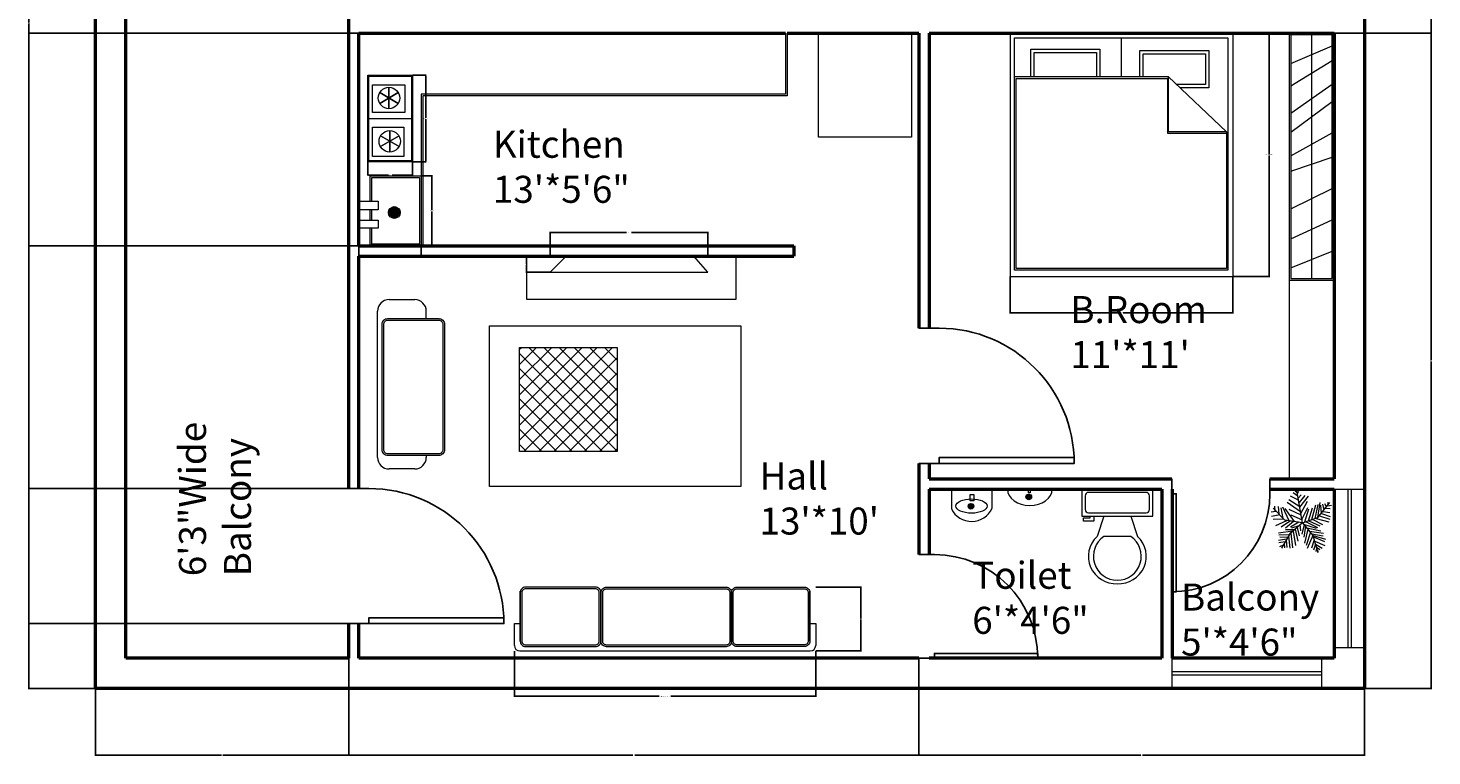
# Model space of a CAD drawing. Units: inches. Extents: x 132738 to 133154, y 138207 to 138641.
# Tile 1 of 2: x 132738 to 133154, y 138207 to 138422. Entities that reach past the tile are written whole.
import ezdxf

# ---------------------------------------------------------------- set-up
doc = ezdxf.new("R2010")
doc.units = ezdxf.units.IN
for name, color, linetype, lineweight in [('A-ANNO-DIMS', 2, 'Continuous', 18), ('A-AREA-IDEN', 7, 'Continuous', 18), ('A-DOOR', 4, 'Continuous', 25), ('A-EQPM', 9, 'Continuous', 18), ('A-FLOR-CASE', 32, 'Continuous', 20), ('A-FLOR-FIXT', 9, 'Continuous', 18), ('A-FURN', 8, 'Continuous', 18), ('A-FURN-PATT', 252, 'Continuous', 13), ('A-GLAZ', 4, 'Continuous', 18), ('A-WALL', 7, 'Continuous', 50), ('L-PLNT', 3, 'Continuous', 13)]:
    doc.layers.add(name, color=color, linetype=linetype, lineweight=lineweight)
doc.styles.get("Standard").update_dxf_attribs({"font": 'arial.ttf'})
doc.dimstyles.get("Standard").update_dxf_attribs({"dimtxt": 0.18, "dimasz": 0.18, "dimexe": 0.18, "dimexo": 0.0625, "dimgap": 0.09, "dimtad": 0, "dimtih": 1, "dimtoh": 1, "dimdec": 4, "dimzin": 0, "dimdsep": 46, "dimtxsty": 'Standard', "dimcen": 0.09, "dimadec": 0, "dimazin": 0, "dimtfac": 1, "dimtdec": 4, "dimtofl": 0, "dimtmove": 0, "dimatfit": 3, "dimfxl": 1, "dimtolj": 1, "dimtzin": 0, "dimarcsym": 0})

# ---------------------------------------------------------------- blocks, each defined once
blk = doc.blocks.new('*U2')
for p, q in [((0, 0), (0, -6)), ((40, 0), (40, -6))]:
    blk.add_line(p, q)
blk.add_lwpolyline([(0, 0), (0, 40), (1.75, 40), (1.75, 0)], close=True)
blk.add_arc((0, 0), 40, 0, 90)
blk = doc.blocks.new('*U4')
for p, q in [((9.5, -6), (9.5, -2)), ((-8, -8.5), (-8, -8)), ((-7, -8), (-7, -9.5)), ((-4, -8), (-6, -14)), ((4, -8), (6, -14)), ((-10, -8.5), (-8, -8.5)), ((-10, -9.5), (-10, -8.5)), ((-7, -9.5), (-10, -9.5)), ((4, -14), (-4, -14))]:
    blk.add_line(p, q)
blk.add_lwpolyline([(10.5, -8), (10.5, 0), (-10.5, 0), (-10.5, -8)], close=True)
for points in [[(-9.5, -2), (-9.5, -6)], [(8.5, -1), (-8.5, -1)], [(-8.5, -7), (8.5, -7)]]:
    blk.add_lwpolyline(points)
for centre, radius, start, end in [((-8.625, -1.875), 0.8839, 81.8699, 188.1301), ((8.625, -1.875), 0.8839, 351.8699, 98.1301), ((-8.625, -6.125), 0.8839, 171.869898, 278.1301), ((8.625, -6.125), 0.8839, 261.8699, 8.1301), ((-0.4772, -19.9188), 8.0953, 133.01722, 273.38), ((0.0374, -19.8731), 7.127, 124.50543, 269.7), ((-0.0373, -19.8731), 7.127, 270.3, 55.4946), ((0.4773, -19.9188), 8.0953, 266.62, 46.9828)]:
    blk.add_arc(centre, radius, start, end)
blk = doc.blocks.new('*U6')
for p, q in [((-8.737, 47.138), (-17.069, 52.711)), ((-10.186, 53.64), (-13.084, 55.962)), ((0, 0), (-10.5, 57)), ((-9.099, 51.782), (-6.563, 55.962)), ((-31.5, 4.5), (-52.5, 25.5)), ((-48.585, 21.131), (-49.309, 29.026)), ((-43.513, 28.561), (-42.427, 15.558)), ((-38.442, 26.239), (-34.819, 7.663)), ((-35.544, 28.097), (-24.314, 3.947)), ((-14.533, 2.09), (-30.834, 25.31)), ((-3.665, 19.273), (-27.574, 35.527)), ((-5.114, 28.097), (-24.676, 40.636)), ((-7.288, 39.707), (-21.778, 46.673)), ((-7.65, 43.423), (-2.578, 49.46)), ((-5.839, 35.992), (4.667, 48.067)), ((-5.114, 27.632), (10.463, 46.673)), ((-2.941, 16.486), (8.652, 37.85)), ((-1.129, 6.734), (9.014, 26.704)), ((10.101, 3.483), (17.708, 26.239)), ((16.259, 5.805), (23.142, 31.348)), ((22.055, 7.198), (27.489, 32.277)), ((27, 9), (48, 36)), ((27.127, 9.056), (31.112, 35.992)), ((31.836, 30.883), (32.561, 16.486)), ((35.096, 32.741), (37.27, 22.524)), ((38.719, 34.134), (41.979, 28.561)), ((40.53, 25.775), (48.862, 24.846)), ((43.791, 29.954), (51.036, 30.883)), ((44.153, 36.456), (45.239, 32.741)), ((-47.498, 19.737), (-55.83, 18.344)), ((-40.615, 13.7), (-55.105, 10.913)), ((-33.37, 6.269), (-52.207, 5.34)), ((-28.299, 3.483), (-47.86, -5.805)), ((-21.416, 3.018), (-38.079, -8.128)), ((0, 0), (-31.5, 4.5)), ((-15.982, 2.09), (-30.11, -9.521)), ((-24.314, 23.917), (-2.941, 13.7)), ((0, 0), (-22.5, -19.5)), ((-6.563, 1.161), (-21.416, -8.128)), ((-20.691, 13.7), (-1.129, 4.876)), ((0, 0), (27, 9)), ((0, 0), (18, -22.5)), ((3.942, 1.625), (11.187, 24.381)), ((6.478, 1.625), (26.04, -8.592)), ((11.187, 3.483), (30.749, -5.805)), ((18.07, 5.805), (35.096, -3.483)), ((24.229, 7.663), (46.688, 1.625)), ((29.662, 12.307), (48.137, 6.269)), ((33.285, 16.486), (48.862, 10.913)), ((36.183, 19.737), (48.137, 17.88)), ((-17.431, -15.094), (-42.789, -18.809)), ((-24.314, -21.596), (-42.427, -22.06)), ((-22.5, -19.5), (-37.5, -45)), ((-15.257, -12.772), (-30.11, -12.772)), ((-25.038, -23.918), (-22.865, -45.281)), ((-20.691, -18.345), (-17.793, -44.352)), ((-6.563, -5.805), (-19.967, -9.985)), ((-17.069, -15.094), (-12.721, -40.172)), ((-13.446, -11.378), (-8.737, -32.741)), ((-9.461, -8.592), (-6.201, -23.453)), ((-4.752, -3.483), (-3.665, -14.629)), ((2.493, -3.019), (-1.491, -20.202)), ((1.769, -2.555), (24.229, -9.521)), ((5.029, -6.27), (2.131, -25.775)), ((9.014, -11.378), (3.58, -35.992)), ((14.085, -16.951), (6.478, -40.172)), ((7.565, -9.056), (32.198, -14.629)), ((18.07, -22.524), (8.289, -45.745)), ((12.274, -15.094), (36.907, -18.809)), ((16.259, -19.738), (36.183, -22.989)), ((18, -22.5), (27, -52.5)), ((18.433, -22.524), (40.53, -29.026)), ((-28.299, -29.026), (-42.789, -31.348)), ((-30.834, -34.135), (-42.427, -35.528)), ((-34.457, -39.708), (-40.978, -42.494)), ((-26.849, -26.24), (-40.253, -25.775)), ((-32.646, -36.921), (-31.921, -44.352)), ((-29.023, -30.884), (-27.936, -43.887)), ((20.244, -30.419), (15.897, -44.816)), ((19.157, -25.311), (38.719, -33.206)), ((22.78, -37.85), (19.519, -48.532)), ((21.331, -32.741), (39.081, -40.636)), ((22.78, -38.314), (34.372, -44.816)), ((24.591, -45.745), (23.142, -50.854)), ((24.591, -43.423), (30.749, -47.603)), ((26.764, -49.925), (28.213, -50.854))]:
    blk.add_line(p, q)
blk = doc.blocks.new('SOFA-THREE-SEAT')
for p, q in [((1.73, 2.94), (1.73, 17.66)), ((87.55, 2.94), (87.55, 17.66)), ((87.55, 9.49), (87.55, 8.16)), ((0, 1.62), (0, 8.16)), ((0, 8.16), (1.73, 8.16)), ((87.55, 8.16), (89.29, 8.16)), ((89.29, 8.16), (89.29, 1.62)), ((1.62, 0), (87.67, 0))]:
    blk.add_line(p, q)
for points in [[(3.35, 1.32), (24.03, 1.32, 0.414214), (25.65, 2.94), (25.65, 17.29, 0.414214), (24.03, 18.91), (3.35, 18.91, 0.414214), (1.73, 17.29), (1.73, 2.94, 0.414214)], [(3.35, 1.82), (24.03, 1.82, 0.414214), (25.15, 2.94), (25.15, 17.29, 0.414214), (24.03, 18.41), (3.35, 18.41, 0.414214), (2.23, 17.29), (2.23, 2.94, 0.414214)], [(62.71, 1.26), (27.29, 1.26, -0.414214), (25.67, 2.88), (25.67, 17.29, -0.414214), (27.29, 18.91), (62.71, 18.91, -0.414214), (64.33, 17.29), (64.33, 2.88, -0.414214)], [(62.71, 1.76), (27.29, 1.76, -0.414214), (26.17, 2.88), (26.17, 17.29, -0.414214), (27.29, 18.41), (62.71, 18.41, -0.414214), (63.83, 17.29), (63.83, 2.88, -0.414214)], [(85.93, 1.32), (65.95, 1.32, -0.414214), (64.33, 2.94), (64.33, 17.29, -0.414214), (65.95, 18.91), (85.93, 18.91, -0.414214), (87.55, 17.29), (87.55, 2.94, -0.414214)], [(85.93, 1.82), (65.95, 1.82, -0.414214), (64.83, 2.94), (64.83, 17.29, -0.414214), (65.95, 18.41), (85.93, 18.41, -0.414214), (87.05, 17.29), (87.05, 2.94, -0.414214)]]:
    blk.add_lwpolyline(points, format="xyb", close=True)
for centre, start, end in [((1.62, 1.62), 180, 270), ((87.67, 1.62), 270, 0)]:
    blk.add_arc(centre, 1.62, start, end)
blk = doc.blocks.new('LOUNGE-CHAIR')
for p, q in [((11.02, 50.13), (3.4, 50.13)), ((0, 3.4), (0, 46.74)), ((14.42, 44.54), (14.42, 46.74)), ((14.42, 4.01), (14.42, 3.4)), ((11.02, 0), (3.4, 0))]:
    blk.add_line(p, q)
for points in [[(1.32, 5.71), (1.32, 42.84, -0.414214), (3.02, 44.54), (18.12, 44.54, -0.414214), (19.82, 42.84), (19.82, 5.71, -0.414214), (18.12, 4.01), (3.02, 4.01, -0.414214)], [(1.82, 5.71), (1.82, 42.84, -0.414214), (3.02, 44.04), (18.12, 44.04, -0.414214), (19.32, 42.84), (19.32, 5.71, -0.414214), (18.12, 4.51), (3.02, 4.51, -0.414214)]]:
    blk.add_lwpolyline(points, format="xyb", close=True)
for centre, start, end in [((3.4, 46.74), 90, 180), ((11.02, 46.74), 0, 90), ((3.4, 3.4), 180, 270), ((11.02, 3.4), 270, 0)]:
    blk.add_arc(centre, 3.4, start, end)
blk = doc.blocks.new('*U18')
blk.add_line((0, 6.36), (0, 0))
blk = doc.blocks.new('*U19')
at = {"color": 0, "linetype": 'ByBlock', "lineweight": -2, "transparency": 16777216}
for p, rotation in [((132078.56, 137807.89), 59.99999999999997), ((132078.56, 137811.07), 119.9999999999999), ((132073.05, 137811.07), 240), ((132073.05, 137807.89), 300), ((132075.81, 137812.66), 180)]:
    blk.add_blockref('*U18', p, dxfattribs=dict(at, rotation=rotation))
blk.add_blockref('*U18', (132075.81, 137806.3), dxfattribs=at)
blk = doc.blocks.new('*U20')
blk.add_line((0, 6.36), (0, 0))
blk = doc.blocks.new('*U21')
at = {"color": 0, "linetype": 'ByBlock', "lineweight": -2, "transparency": 16777216}
for p, rotation in [((132078.34, 137820.7), 59.99999999999997), ((132078.34, 137823.88), 119.9999999999999), ((132072.84, 137823.88), 240), ((132072.84, 137820.7), 300), ((132075.59, 137825.47), 180)]:
    blk.add_blockref('*U20', p, dxfattribs=dict(at, rotation=rotation))
blk.add_blockref('*U20', (132075.59, 137819.12), dxfattribs=at)
blk = doc.blocks.new('COOKTOP-TWO-BURNER')
blk.add_line((0, 12.86), (13.26, 12.86))
for points in [[(0, 25.73), (13.26, 25.73), (13.26, 0), (0, 0)], [(0.3, 25.43), (12.96, 25.43), (12.96, 0.3), (0.3, 0.3)], [(1.41, 22.8), (10.98, 22.8), (10.98, 14.61), (1.41, 14.61)], [(1.41, 10.35), (10.68, 10.35), (10.68, 1.58), (1.41, 1.58)]]:
    blk.add_lwpolyline(points, close=True)
for centre in [(6.25, 18.94), (6.47, 6.13)]:
    blk.add_circle(centre, 3.18)
for name in ['*U21', '*U19']:
    blk.add_blockref(name, (-132069.34, -137803.35))
blk = doc.blocks.new('*U16')
blk.add_line((0, 3.48), (0, 0))
blk = doc.blocks.new('*U17')
at = {"color": 0, "linetype": 'ByBlock', "lineweight": -2, "transparency": 16777216}
for p, rotation in [((132078.22, 137785.99), 90), ((132074.74, 137785.99), 270), ((132078.13, 137785.45), 71.99999999999999), ((132078.13, 137786.53), 108), ((132074.83, 137786.53), 252), ((132074.83, 137785.45), 288), ((132077.89, 137784.97), 53.99999999999998), ((132077.89, 137787.01), 126), ((132075.08, 137787.01), 234), ((132075.08, 137784.97), 306), ((132077.5, 137784.59), 35.99999999999999), ((132077.5, 137787.4), 144), ((132075.46, 137787.4), 216), ((132075.46, 137784.59), 323.9999999999999), ((132077.02, 137784.34), 17.99999999999998), ((132077.02, 137787.64), 162), ((132075.95, 137787.64), 198), ((132075.95, 137784.34), 342), ((132076.48, 137787.73), 180)]:
    blk.add_blockref('*U16', p, dxfattribs=dict(at, rotation=rotation))
blk.add_blockref('*U16', (132076.48, 137784.25), dxfattribs=at)
blk = doc.blocks.new('SINK-KITCHEN')
blk.add_line((3.38, 20.8), (18.5, 20.8))
for points in [[(3.38, 13.25), (3.38, 20.8), (18.5, 20.8), (18.5, 0), (3.38, 0), (3.38, 5.25)], [(3.88, 13.25), (3.88, 20.3), (18, 20.3), (18, 0.5), (3.88, 0.5), (3.88, 5.25)], [(3.38, 7.61), (3.38, 10.65)], [(3.88, 7.61), (3.88, 10.65)]]:
    blk.add_lwpolyline(points)
for points in [[(0, 13.25), (5.74, 13.25), (5.74, 10.65), (0, 10.65)], [(0, 7.61), (5.74, 7.61), (5.74, 5.25), (0, 5.25)]]:
    blk.add_lwpolyline(points, close=True)
blk.add_circle((10.52, 9.9), 1.74)
blk.add_blockref('*U17', (-132065.96, -137776.09))
blk = doc.blocks.new('*U9')
blk.add_line((0, 1.68), (0, 0))
blk = doc.blocks.new('*U10')
at = {"color": 0, "linetype": 'ByBlock', "lineweight": -2, "transparency": 16777216}
for p, rotation in [((132265.47, 137716.61), 90), ((132263.79, 137716.61), 270), ((132265.42, 137716.35), 71.99999999999999), ((132265.42, 137716.87), 108), ((132263.83, 137716.87), 252), ((132263.83, 137716.35), 288), ((132265.31, 137716.12), 53.99999999999998), ((132265.31, 137717.1), 126), ((132263.95, 137717.1), 234), ((132263.95, 137716.12), 306), ((132265.12, 137715.93), 35.99999999999999), ((132265.12, 137717.29), 144), ((132264.13, 137717.29), 216), ((132264.13, 137715.93), 324), ((132264.89, 137715.81), 17.99999999999997), ((132264.89, 137717.41), 162), ((132264.37, 137717.41), 197.9999999999999), ((132264.37, 137715.81), 342), ((132264.63, 137717.45), 180)]:
    blk.add_blockref('*U9', p, dxfattribs=dict(at, rotation=rotation))
blk.add_blockref('*U9', (132264.63, 137715.77), dxfattribs=at)
blk = doc.blocks.new('BASIN-OVAL')
blk.add_lwpolyline([(6.22, 4.85), (6.68, 4.85), (6.68, 3.77), (6.22, 3.77)], close=True)
blk.add_circle((6.31, 2.53), 0.838)
blk.add_ellipse((6.62, 4.85), major_axis=(6.62, 0), ratio=0.732474, start_param=3.141593, end_param=6.283185)
blk.add_blockref('*U10', (-132258.32, -137714.08))
blk = doc.blocks.new('*U11')
blk.add_line((0, 1.68), (0, 0))
blk = doc.blocks.new('*U12')
at = {"color": 0, "linetype": 'ByBlock', "lineweight": -2, "transparency": 16777216}
for p, rotation in [((132265.47, 137716.61), 90), ((132263.79, 137716.61), 270), ((132265.42, 137716.35), 71.99999999999999), ((132265.42, 137716.87), 108), ((132263.83, 137716.87), 252), ((132263.83, 137716.35), 288), ((132265.31, 137716.12), 53.99999999999998), ((132265.31, 137717.1), 126), ((132263.95, 137717.1), 234), ((132263.95, 137716.12), 306), ((132265.12, 137715.93), 35.99999999999999), ((132265.12, 137717.29), 144), ((132264.13, 137717.29), 216), ((132264.13, 137715.93), 324), ((132264.89, 137715.81), 17.99999999999997), ((132264.89, 137717.41), 162), ((132264.37, 137717.41), 197.9999999999999), ((132264.37, 137715.81), 342), ((132264.63, 137717.45), 180)]:
    blk.add_blockref('*U11', p, dxfattribs=dict(at, rotation=rotation))
blk.add_blockref('*U11', (132264.63, 137715.77), dxfattribs=at)
blk = doc.blocks.new('BASIN-WALL')
for p, q in [((0, 9.56), (0, 3.71)), ((12.04, 3.88), (12.04, 9.56))]:
    blk.add_line(p, q)
blk.add_lwpolyline([(5.55, 7.94), (6.68, 7.94), (6.68, 6.05), (5.55, 6.05)], close=True)
blk.add_circle((5.81, 4.48), 0.838)
blk.add_arc((5.98, 6.67), 6.67, 206.3567, 335.2907)
blk.add_ellipse((5.98, 4.55), major_axis=(4.63, 0), ratio=0.457552)
blk.add_blockref('*U12', (-132258.82, -137712.13))
blk = doc.blocks.new('BED-DOUBLE')
for p, q in [((0, 72), (0, 0)), ((66, 72), (66, 0)), ((1.29, 59.19), (46.8, 59.19)), ((46.61, 58.57), (46.61, 42.39)), ((46.8, 59.19), (64.12, 42.79)), ((46.8, 59.19), (46.8, 42.79)), ((46.61, 42.39), (64.12, 42.39)), ((64.12, 42.79), (46.8, 42.79)), ((0, 0), (66, 0))]:
    blk.add_line(p, q)
blk.add_lwpolyline([(1.29, 70.58), (64.54, 70.58), (64.54, 1.81), (1.29, 1.81)], close=True)
blk.add_lwpolyline([(64.12, 42.79), (64.12, 2.3), (1.76, 2.3), (1.76, 58.57), (46.61, 58.57)])
blk = doc.blocks.new('WARDROBE')
for p, q in [((6.65, 72.63), (6.65, 0.5)), ((0.5, 64.18), (12.79, 69.35)), ((0.5, 57.53), (12.79, 65.06)), ((0.5, 49.42), (12.79, 58.04)), ((0.5, 43.85), (12.79, 52.9)), ((0.5, 36.84), (12.79, 43.67)), ((0.5, 32.25), (12.79, 36.4)), ((0.5, 21.15), (12.79, 27.18)), ((0.5, 12.28), (12.79, 17.88)), ((0.5, 3.64), (12.79, 8.6))]:
    blk.add_line(p, q)
for points in [[(13.29, 73.13), (0, 73.13), (0, 0), (13.29, 0)], [(12.79, 72.63), (0.5, 72.63), (0.5, 0.5), (12.79, 0.5)]]:
    blk.add_lwpolyline(points, close=True)
blk = doc.blocks.new('TV-FLATSCREEN')
for p, q in [((4.76, 4.76), (0, 0)), ((46.75, 0), (42.54, 4.76)), ((0, 0), (46.75, 0))]:
    blk.add_line(p, q)
blk = doc.blocks.new('*D34')
at = {"layer": 'A-ANNO-DIMS', "color": 0, "lineweight": -2, "transparency": 16777216}
for p, q in [((132882.07, 138237.94), (132882.07, 138224.43)), ((132971.36, 138237.94), (132971.36, 138224.43)), ((132882.25, 138224.61), (132924.97, 138224.61)), ((132971.18, 138224.61), (132928.45, 138224.61))]:
    blk.add_line(p, q, dxfattribs=at)
at = {"layer": 'A-ANNO-DIMS', "color": 0, "transparency": 16777216}
for points in [[(132882.25, 138224.64), (132882.25, 138224.58), (132882.07, 138224.61)], [(132971.18, 138224.64), (132971.18, 138224.58), (132971.36, 138224.61)]]:
    blk.add_solid(points, dxfattribs=at)
at = {"layer": 'Defpoints', "color": 0, "transparency": 16777216}
for p in [(132882.07, 138238), (132971.36, 138238), (132971.36, 138224.61)]:
    blk.add_point(p, dxfattribs=at)
at = {"layer": 'A-ANNO-DIMS', "color": 0, "transparency": 16777216, "insert": (132926.71, 138224.61), "char_height": 0.18, "attachment_point": 5}
blk.add_mtext('\\A1;THREE-SEAT SOFA 89 TYP.', dxfattribs=at)
blk = doc.blocks.new('*D35')
at = {"layer": 'A-ANNO-DIMS', "color": 0, "lineweight": -2, "transparency": 16777216}
for p, q in [((132971.42, 138256.91), (132984.93, 138256.91)), ((132984.75, 138256.73), (132984.75, 138247.64)), ((132984.75, 138238.18), (132984.75, 138247.28)), ((132971.42, 138238), (132984.93, 138238))]:
    blk.add_line(p, q, dxfattribs=at)
at = {"layer": 'A-ANNO-DIMS', "color": 0, "transparency": 16777216}
for points in [[(132984.72, 138256.73), (132984.78, 138256.73), (132984.75, 138256.91)], [(132984.72, 138238.18), (132984.78, 138238.18), (132984.75, 138238)]]:
    blk.add_solid(points, dxfattribs=at)
at = {"layer": 'Defpoints', "color": 0, "transparency": 16777216}
for p in [(132971.36, 138256.91), (132984.75, 138256.91), (132971.36, 138238)]:
    blk.add_point(p, dxfattribs=at)
at = {"layer": 'A-ANNO-DIMS', "color": 0, "transparency": 16777216, "insert": (132984.75, 138247.46), "char_height": 0.18, "attachment_point": 5}
blk.add_mtext('\\A1;19 TYP.', dxfattribs=at)
blk = doc.blocks.new('*D38')
at = {"layer": 'A-ANNO-DIMS', "color": 0, "lineweight": -2, "transparency": 16777216}
for p, q in [((132851.98, 138408.51), (132855.96, 138408.51)), ((132855.78, 138408.33), (132855.78, 138395.83)), ((132855.78, 138382.96), (132855.78, 138395.46)), ((132851.98, 138382.78), (132855.96, 138382.78))]:
    blk.add_line(p, q, dxfattribs=at)
at = {"layer": 'A-ANNO-DIMS', "color": 0, "transparency": 16777216}
for points in [[(132855.75, 138408.33), (132855.81, 138408.33), (132855.78, 138408.51)], [(132855.75, 138382.96), (132855.81, 138382.96), (132855.78, 138382.78)]]:
    blk.add_solid(points, dxfattribs=at)
at = {"layer": 'Defpoints', "color": 0, "transparency": 16777216}
for p in [(132851.92, 138408.51), (132855.78, 138408.51), (132851.92, 138382.78)]:
    blk.add_point(p, dxfattribs=at)
at = {"layer": 'A-ANNO-DIMS', "color": 0, "transparency": 16777216, "insert": (132855.78, 138395.64), "char_height": 0.18, "attachment_point": 5}
blk.add_mtext('\\A1;HOB 26 TYP.', dxfattribs=at)
blk = doc.blocks.new('*D39')
at = {"layer": 'A-ANNO-DIMS', "color": 0, "lineweight": -2, "transparency": 16777216}
for p, q in [((132838.66, 138382.72), (132838.66, 138378.74)), ((132851.92, 138382.72), (132851.92, 138378.74)), ((132838.84, 138378.92), (132844.77, 138378.92)), ((132851.74, 138378.92), (132845.81, 138378.92))]:
    blk.add_line(p, q, dxfattribs=at)
at = {"layer": 'A-ANNO-DIMS', "color": 0, "transparency": 16777216}
for points in [[(132838.84, 138378.95), (132838.84, 138378.89), (132838.66, 138378.92)], [(132851.74, 138378.95), (132851.74, 138378.89), (132851.92, 138378.92)]]:
    blk.add_solid(points, dxfattribs=at)
at = {"layer": 'Defpoints', "color": 0, "transparency": 16777216}
for p in [(132838.66, 138382.78), (132851.92, 138382.78), (132851.92, 138378.92)]:
    blk.add_point(p, dxfattribs=at)
at = {"layer": 'A-ANNO-DIMS', "color": 0, "transparency": 16777216, "insert": (132845.29, 138378.92), "char_height": 0.18, "attachment_point": 5}
blk.add_mtext('\\A1;13 TYP.', dxfattribs=at)
blk = doc.blocks.new('*D40')
at = {"layer": 'A-ANNO-DIMS', "color": 0, "lineweight": -2, "transparency": 16777216}
for p, q in [((132854.52, 138378.73), (132857.76, 138378.73)), ((132857.58, 138378.55), (132857.58, 138368.51)), ((132857.58, 138358.1), (132857.58, 138368.14)), ((132854.52, 138357.92), (132857.76, 138357.92))]:
    blk.add_line(p, q, dxfattribs=at)
at = {"layer": 'A-ANNO-DIMS', "color": 0, "transparency": 16777216}
for points in [[(132857.55, 138378.55), (132857.61, 138378.55), (132857.58, 138378.73)], [(132857.55, 138358.1), (132857.61, 138358.1), (132857.58, 138357.92)]]:
    blk.add_solid(points, dxfattribs=at)
at = {"layer": 'Defpoints', "color": 0, "transparency": 16777216}
for p in [(132854.46, 138378.73), (132857.58, 138378.73), (132854.46, 138357.92)]:
    blk.add_point(p, dxfattribs=at)
at = {"layer": 'A-ANNO-DIMS', "color": 0, "transparency": 16777216, "insert": (132857.58, 138368.32), "char_height": 0.18, "attachment_point": 5}
blk.add_mtext('\\A1;SINK 21 TYP.', dxfattribs=at)
blk = doc.blocks.new('*D41')
at = {"layer": 'A-ANNO-DIMS', "color": 0, "lineweight": -2, "transparency": 16777216}
for p, q in [((132835.96, 138357.86), (132835.96, 138354.62)), ((132854.46, 138357.86), (132854.46, 138354.62)), ((132836.14, 138354.8), (132844.69, 138354.8)), ((132854.28, 138354.8), (132845.73, 138354.8))]:
    blk.add_line(p, q, dxfattribs=at)
at = {"layer": 'A-ANNO-DIMS', "color": 0, "transparency": 16777216}
for points in [[(132836.14, 138354.83), (132836.14, 138354.77), (132835.96, 138354.8)], [(132854.28, 138354.83), (132854.28, 138354.77), (132854.46, 138354.8)]]:
    blk.add_solid(points, dxfattribs=at)
at = {"layer": 'Defpoints', "color": 0, "transparency": 16777216}
for p in [(132835.96, 138357.92), (132854.46, 138357.92), (132854.46, 138354.8)]:
    blk.add_point(p, dxfattribs=at)
at = {"layer": 'A-ANNO-DIMS', "color": 0, "transparency": 16777216, "insert": (132845.21, 138354.8), "char_height": 0.18, "attachment_point": 5}
blk.add_mtext('\\A1;18 TYP.', dxfattribs=at)
blk = doc.blocks.new('*D46')
at = {"layer": 'A-ANNO-DIMS', "color": 0, "lineweight": -2, "transparency": 16777216}
for p, q in [((133095.02, 138420.92), (133105.94, 138420.92)), ((133105.76, 138420.74), (133105.76, 138385.11)), ((133105.76, 138349.1), (133105.76, 138384.74)), ((133095.02, 138348.92), (133105.94, 138348.92))]:
    blk.add_line(p, q, dxfattribs=at)
at = {"layer": 'A-ANNO-DIMS', "color": 0, "transparency": 16777216}
for points in [[(133105.73, 138420.74), (133105.79, 138420.74), (133105.76, 138420.92)], [(133105.73, 138349.1), (133105.79, 138349.1), (133105.76, 138348.92)]]:
    blk.add_solid(points, dxfattribs=at)
at = {"layer": 'Defpoints', "color": 0, "transparency": 16777216}
for p in [(133094.96, 138420.92), (133105.76, 138420.92), (133094.96, 138348.92)]:
    blk.add_point(p, dxfattribs=at)
at = {"layer": 'A-ANNO-DIMS', "color": 0, "transparency": 16777216, "insert": (133105.76, 138384.92), "char_height": 0.18, "attachment_point": 5}
blk.add_mtext('\\A1;DOUBLE BED 72 TYP.', dxfattribs=at)
blk = doc.blocks.new('*D47')
at = {"layer": 'A-ANNO-DIMS', "color": 0, "lineweight": -2, "transparency": 16777216}
for p, q in [((133028.96, 138348.86), (133028.96, 138337.94)), ((133094.96, 138348.86), (133094.96, 138337.94)), ((133029.14, 138338.12), (133061.43, 138338.12)), ((133094.78, 138338.12), (133062.49, 138338.12))]:
    blk.add_line(p, q, dxfattribs=at)
at = {"layer": 'A-ANNO-DIMS', "color": 0, "transparency": 16777216}
for points in [[(133029.14, 138338.15), (133029.14, 138338.09), (133028.96, 138338.12)], [(133094.78, 138338.15), (133094.78, 138338.09), (133094.96, 138338.12)]]:
    blk.add_solid(points, dxfattribs=at)
at = {"layer": 'Defpoints', "color": 0, "transparency": 16777216}
for p in [(133028.96, 138348.92), (133094.96, 138348.92), (133094.96, 138338.12)]:
    blk.add_point(p, dxfattribs=at)
at = {"layer": 'A-ANNO-DIMS', "color": 0, "transparency": 16777216, "insert": (133061.96, 138338.12), "char_height": 0.18, "attachment_point": 5}
blk.add_mtext('\\A1;66 TYP.', dxfattribs=at)
blk = doc.blocks.new('*D50')
at = {"layer": 'A-ANNO-DIMS', "color": 0, "lineweight": -2, "transparency": 16777216}
for p, q in [((132892.69, 138354.99), (132892.69, 138362.12)), ((132892.87, 138361.94), (132915.33, 138361.94)), ((132939.25, 138361.94), (132916.79, 138361.94)), ((132939.43, 138354.99), (132939.43, 138362.12))]:
    blk.add_line(p, q, dxfattribs=at)
at = {"layer": 'A-ANNO-DIMS', "color": 0, "transparency": 16777216}
for points in [[(132892.87, 138361.97), (132892.87, 138361.91), (132892.69, 138361.94)], [(132939.25, 138361.97), (132939.25, 138361.91), (132939.43, 138361.94)]]:
    blk.add_solid(points, dxfattribs=at)
at = {"layer": 'Defpoints', "color": 0, "transparency": 16777216}
for p in [(132939.43, 138361.94), (132892.69, 138354.92), (132939.43, 138354.92)]:
    blk.add_point(p, dxfattribs=at)
at = {"layer": 'A-ANNO-DIMS', "color": 0, "transparency": 16777216, "insert": (132916.06, 138361.94), "char_height": 0.18, "attachment_point": 5}
blk.add_mtext('\\A1;TV 47 TYP.', dxfattribs=at)
blk = doc.blocks.new('*D51')
at = {"layer": 'A-ANNO-DIMS', "color": 0, "lineweight": -2, "transparency": 16777216}
for p, q in [((132892.62, 138354.92), (132885.49, 138354.92)), ((132885.67, 138354.74), (132885.67, 138352.72)), ((132885.67, 138350.34), (132885.67, 138352.36)), ((132892.62, 138350.16), (132885.49, 138350.16))]:
    blk.add_line(p, q, dxfattribs=at)
at = {"layer": 'A-ANNO-DIMS', "color": 0, "transparency": 16777216}
for points in [[(132885.64, 138354.74), (132885.7, 138354.74), (132885.67, 138354.92)], [(132885.64, 138350.34), (132885.7, 138350.34), (132885.67, 138350.16)]]:
    blk.add_solid(points, dxfattribs=at)
at = {"layer": 'Defpoints', "color": 0, "transparency": 16777216}
for p in [(132885.67, 138354.92), (132892.69, 138354.92), (132892.69, 138350.16)]:
    blk.add_point(p, dxfattribs=at)
at = {"layer": 'A-ANNO-DIMS', "color": 0, "transparency": 16777216, "insert": (132885.67, 138352.54), "char_height": 0.18, "attachment_point": 5}
blk.add_mtext('\\A1;5 TYP.', dxfattribs=at)
blk = doc.blocks.new('*D53')
at = {"layer": 'A-ANNO-DIMS', "color": 0, "lineweight": -2, "transparency": 16777216}
for p, q in [((132757.9, 138620.92), (132737.98, 138620.92)), ((132738.16, 138620.74), (132738.16, 138424.1)), ((132738.16, 138227.1), (132738.16, 138423.74)), ((132757.9, 138226.92), (132737.98, 138226.92))]:
    blk.add_line(p, q, dxfattribs=at)
at = {"layer": 'A-ANNO-DIMS', "color": 0, "transparency": 16777216}
for points in [[(132738.13, 138620.74), (132738.19, 138620.74), (132738.16, 138620.92)], [(132738.13, 138227.1), (132738.19, 138227.1), (132738.16, 138226.92)]]:
    blk.add_solid(points, dxfattribs=at)
at = {"layer": 'Defpoints', "color": 0, "transparency": 16777216}
for p in [(132738.16, 138620.92), (132757.96, 138620.92), (132757.96, 138226.92)]:
    blk.add_point(p, dxfattribs=at)
at = {"layer": 'A-ANNO-DIMS', "color": 0, "transparency": 16777216, "insert": (132738.16, 138423.92), "char_height": 0.18, "attachment_point": 5}
blk.add_mtext('\\A1;394', dxfattribs=at)
blk = doc.blocks.new('*D54')
at = {"layer": 'A-ANNO-DIMS', "color": 0, "lineweight": -2, "transparency": 16777216}
for p, q in [((132832.96, 138235.86), (132832.96, 138206.94)), ((132757.96, 138226.86), (132757.96, 138206.94)), ((132758.14, 138207.12), (132795.24, 138207.12)), ((132832.78, 138207.12), (132795.68, 138207.12))]:
    blk.add_line(p, q, dxfattribs=at)
at = {"layer": 'A-ANNO-DIMS', "color": 0, "transparency": 16777216}
for points in [[(132758.14, 138207.15), (132758.14, 138207.09), (132757.96, 138207.12)], [(132832.78, 138207.15), (132832.78, 138207.09), (132832.96, 138207.12)]]:
    blk.add_solid(points, dxfattribs=at)
at = {"layer": 'Defpoints', "color": 0, "transparency": 16777216}
for p in [(132832.96, 138235.92), (132757.96, 138226.92), (132832.96, 138207.12)]:
    blk.add_point(p, dxfattribs=at)
at = {"layer": 'A-ANNO-DIMS', "color": 0, "transparency": 16777216, "insert": (132795.46, 138207.12), "char_height": 0.18, "attachment_point": 5}
blk.add_mtext('\\A1;75', dxfattribs=at)
blk = doc.blocks.new('*D55')
at = {"layer": 'A-ANNO-DIMS', "color": 0, "lineweight": -2, "transparency": 16777216}
for p, q in [((132832.96, 138235.86), (132832.96, 138206.94)), ((133001.96, 138235.86), (133001.96, 138206.94)), ((132833.14, 138207.12), (132917.18, 138207.12)), ((133001.78, 138207.12), (132917.74, 138207.12))]:
    blk.add_line(p, q, dxfattribs=at)
at = {"layer": 'A-ANNO-DIMS', "color": 0, "transparency": 16777216}
for points in [[(132833.14, 138207.15), (132833.14, 138207.09), (132832.96, 138207.12)], [(133001.78, 138207.15), (133001.78, 138207.09), (133001.96, 138207.12)]]:
    blk.add_solid(points, dxfattribs=at)
at = {"layer": 'Defpoints', "color": 0, "transparency": 16777216}
for p in [(132832.96, 138235.92), (133001.96, 138235.92), (133001.96, 138207.12)]:
    blk.add_point(p, dxfattribs=at)
at = {"layer": 'A-ANNO-DIMS', "color": 0, "transparency": 16777216, "insert": (132917.46, 138207.12), "char_height": 0.18, "attachment_point": 5}
blk.add_mtext('\\A1;169', dxfattribs=at)
blk = doc.blocks.new('*D56')
at = {"layer": 'A-ANNO-DIMS', "color": 0, "lineweight": -2, "transparency": 16777216}
for p, q in [((133001.96, 138235.86), (133001.96, 138206.94)), ((133133.96, 138226.86), (133133.96, 138206.94)), ((133002.14, 138207.12), (133067.68, 138207.12)), ((133133.78, 138207.12), (133068.24, 138207.12))]:
    blk.add_line(p, q, dxfattribs=at)
at = {"layer": 'A-ANNO-DIMS', "color": 0, "transparency": 16777216}
for points in [[(133002.14, 138207.15), (133002.14, 138207.09), (133001.96, 138207.12)], [(133133.78, 138207.15), (133133.78, 138207.09), (133133.96, 138207.12)]]:
    blk.add_solid(points, dxfattribs=at)
at = {"layer": 'Defpoints', "color": 0, "transparency": 16777216}
for p in [(133001.96, 138235.92), (133133.96, 138226.92), (133133.96, 138207.12)]:
    blk.add_point(p, dxfattribs=at)
at = {"layer": 'A-ANNO-DIMS', "color": 0, "transparency": 16777216, "insert": (133067.96, 138207.12), "char_height": 0.18, "attachment_point": 5}
blk.add_mtext('\\A1;132', dxfattribs=at)
blk = doc.blocks.new('*D57')
at = {"layer": 'A-ANNO-DIMS', "color": 0, "lineweight": -2, "transparency": 16777216}
for p, q in [((133125.02, 138420.92), (133153.95, 138420.92)), ((133153.77, 138420.74), (133153.77, 138324.1)), ((133153.77, 138227.1), (133153.77, 138323.74)), ((133134.02, 138226.92), (133153.95, 138226.92))]:
    blk.add_line(p, q, dxfattribs=at)
at = {"layer": 'A-ANNO-DIMS', "color": 0, "transparency": 16777216}
for points in [[(133153.74, 138420.74), (133153.8, 138420.74), (133153.77, 138420.92)], [(133153.74, 138227.1), (133153.8, 138227.1), (133153.77, 138226.92)]]:
    blk.add_solid(points, dxfattribs=at)
at = {"layer": 'Defpoints', "color": 0, "transparency": 16777216}
for p in [(133124.96, 138420.92), (133153.77, 138420.92), (133133.96, 138226.92)]:
    blk.add_point(p, dxfattribs=at)
at = {"layer": 'A-ANNO-DIMS', "color": 0, "transparency": 16777216, "insert": (133153.77, 138323.92), "char_height": 0.18, "attachment_point": 5}
blk.add_mtext('\\A1;194', dxfattribs=at)
blk = doc.blocks.new('*D58')
at = {"layer": 'A-ANNO-DIMS', "color": 0, "lineweight": -2, "transparency": 16777216}
for p, q in [((132835.9, 138420.92), (132737.98, 138420.92)), ((132738.16, 138420.74), (132738.16, 138389.6)), ((132738.16, 138358.1), (132738.16, 138389.24)), ((132835.9, 138357.92), (132737.98, 138357.92))]:
    blk.add_line(p, q, dxfattribs=at)
at = {"layer": 'A-ANNO-DIMS', "color": 0, "transparency": 16777216}
for points in [[(132738.13, 138420.74), (132738.19, 138420.74), (132738.16, 138420.92)], [(132738.13, 138358.1), (132738.19, 138358.1), (132738.16, 138357.92)]]:
    blk.add_solid(points, dxfattribs=at)
at = {"layer": 'Defpoints', "color": 0, "transparency": 16777216}
for p in [(132738.16, 138420.92), (132835.96, 138420.92), (132835.96, 138357.92)]:
    blk.add_point(p, dxfattribs=at)
at = {"layer": 'A-ANNO-DIMS', "color": 0, "transparency": 16777216, "insert": (132738.16, 138389.42), "char_height": 0.18, "attachment_point": 5}
blk.add_mtext('\\A1;63', dxfattribs=at)
blk = doc.blocks.new('*D59')
at = {"layer": 'A-ANNO-DIMS', "color": 0, "lineweight": -2, "transparency": 16777216}
for p, q in [((132832.9, 138286.11), (132737.98, 138286.11)), ((132738.16, 138285.93), (132738.16, 138266.29)), ((132738.16, 138246.29), (132738.16, 138265.92)), ((132832.9, 138246.11), (132737.98, 138246.11))]:
    blk.add_line(p, q, dxfattribs=at)
at = {"layer": 'A-ANNO-DIMS', "color": 0, "transparency": 16777216}
for points in [[(132738.13, 138285.93), (132738.19, 138285.93), (132738.16, 138286.11)], [(132738.13, 138246.29), (132738.19, 138246.29), (132738.16, 138246.11)]]:
    blk.add_solid(points, dxfattribs=at)
at = {"layer": 'Defpoints', "color": 0, "transparency": 16777216}
for p in [(132738.16, 138286.11), (132832.96, 138286.11), (132832.96, 138246.11)]:
    blk.add_point(p, dxfattribs=at)
at = {"layer": 'A-ANNO-DIMS', "color": 0, "transparency": 16777216, "insert": (132738.16, 138266.11), "char_height": 0.18, "attachment_point": 5}
blk.add_mtext('\\A1;40', dxfattribs=at)
blk = doc.blocks.new('*D61')
at = {"layer": 'A-ANNO-DIMS', "color": 0, "lineweight": -2, "transparency": 16777216}
for p, q in [((133125.02, 138491.92), (133153.95, 138491.92)), ((133153.77, 138491.74), (133153.77, 138456.6)), ((133153.77, 138421.1), (133153.77, 138456.24)), ((133125.02, 138420.92), (133153.95, 138420.92))]:
    blk.add_line(p, q, dxfattribs=at)
at = {"layer": 'A-ANNO-DIMS', "color": 0, "transparency": 16777216}
for points in [[(133153.74, 138491.74), (133153.8, 138491.74), (133153.77, 138491.92)], [(133153.74, 138421.1), (133153.8, 138421.1), (133153.77, 138420.92)]]:
    blk.add_solid(points, dxfattribs=at)
at = {"layer": 'Defpoints', "color": 0, "transparency": 16777216}
for p in [(133124.96, 138491.92), (133153.77, 138491.92), (133124.96, 138420.92)]:
    blk.add_point(p, dxfattribs=at)
at = {"layer": 'A-ANNO-DIMS', "color": 0, "transparency": 16777216, "insert": (133153.77, 138456.42), "char_height": 0.18, "attachment_point": 5}
blk.add_mtext('\\A1;71', dxfattribs=at)

msp = doc.modelspace()

# ---------------------------------------------------------------- hatches: boundary and pattern name
at = {"layer": 'A-FURN-PATT'}
h = msp.add_hatch(dxfattribs=at)
h.set_pattern_fill('ANSI37', color=256)
h.set_pattern_definition([(45, (769.9685, 583.0495), (-2.24506403, 2.24506403), []), (135, (769.9685, 583.0495), (-2.24506403, -2.24506403), [])])
h.paths.add_polyline_path([(132883.613, 138327.862), (132912.513, 138327.862), (132912.513, 138297.088), (132883.613, 138297.088)])

# ---------------------------------------------------------------- linework, layer by layer
at = {"layer": 'A-EQPM'}
msp.add_lwpolyline([(132972.224, 138420.923), (132999.748, 138420.923), (132999.748, 138390.147), (132972.224, 138390.147)], close=True, dxfattribs=at)
at = {"layer": 'A-FLOR-CASE'}
for p, q in [((132962.423, 138420.923), (132962.423, 138402.865)), ((132962.923, 138420.923), (132962.923, 138402.365)), ((133118.314, 138420.423), (133118.314, 138348.292)), ((132962.423, 138402.865), (132854.448, 138402.865)), ((132854.448, 138402.865), (132854.448, 138378.592)), ((132962.923, 138402.365), (132854.948, 138402.365)), ((132854.948, 138402.365), (132854.948, 138378.092)), ((132854.948, 138378.092), (132854.948, 138357.923)), ((133111.667, 138347.792), (133111.667, 138294.171)), ((133111.667, 138294.171), (133111.667, 138288.923))]:
    msp.add_line(p, q, dxfattribs=at)
at = {"layer": 'A-FURN'}
msp.add_line((133061.88, 138419.508), (133061.88, 138408.112), dxfattribs=at)
for points in [[(133035.124, 138408.112), (133035.124, 138416.167), (133055.597, 138416.167), (133055.597, 138408.112)], [(133036.124, 138408.112), (133036.124, 138415.167), (133054.597, 138415.167), (133054.597, 138408.112)], [(133067.419, 138408.112), (133067.419, 138415.838), (133087.892, 138415.838), (133087.892, 138404.716), (133079.345, 138404.716)], [(133068.419, 138408.112), (133068.419, 138414.838), (133086.892, 138414.838), (133086.892, 138405.716), (133078.288, 138405.716)]]:
    msp.add_lwpolyline(points, dxfattribs=at)
for points in [[(132885.796, 138354.923), (132947.711, 138354.923), (132947.711, 138342.025), (132885.796, 138342.025)], [(132874.721, 138334.316), (132949.136, 138334.316), (132949.136, 138286.68), (132874.721, 138286.68)], [(132883.613, 138327.862), (132912.513, 138327.862), (132912.513, 138297.088), (132883.613, 138297.088)]]:
    msp.add_lwpolyline(points, close=True, dxfattribs=at)
at = {"layer": 'A-GLAZ'}
for p, q in [((133129.023, 138285.916), (133129.023, 138239.068)), ((133130.023, 138285.914), (133130.023, 138239.068)), ((133124.961, 138239.068), (133133.961, 138239.068)), ((133121.226, 138235.923), (133121.226, 138226.923)), ((133121.226, 138231.861), (133076.961, 138231.861)), ((133121.226, 138230.861), (133076.961, 138230.861))]:
    msp.add_line(p, q, dxfattribs=at)
for points in [[(133124.961, 138235.923), (133124.961, 138285.923), (133133.961, 138285.907), (133133.961, 138235.923)], [(133133.961, 138226.923), (133076.961, 138226.923), (133076.961, 138235.923), (133124.961, 138235.923)]]:
    msp.add_lwpolyline(points, dxfattribs=at)
at = {"layer": 'A-WALL'}
for p, q in [((132757.961, 138226.923), (132757.961, 138620.923)), ((133133.961, 138620.923), (133133.961, 138226.923)), ((132766.961, 138235.923), (132766.961, 138611.923)), ((132832.961, 138286.105), (132832.961, 138434.453)), ((132835.961, 138420.923), (132962.423, 138420.923)), ((132835.961, 138378.592), (132835.961, 138420.923)), ((132962.923, 138420.923), (133001.961, 138420.923)), ((133001.961, 138420.923), (133001.961, 138333.554)), ((133004.961, 138420.923), (133124.961, 138420.923)), ((133004.961, 138420.923), (133004.961, 138333.554)), ((133124.961, 138420.923), (133124.961, 138288.923)), ((132835.961, 138357.923), (132835.961, 138378.592)), ((132835.961, 138357.923), (132964.885, 138357.923)), ((132964.885, 138357.923), (132964.885, 138354.923)), ((132835.961, 138354.923), (132964.885, 138354.923)), ((132835.961, 138286.105), (132835.961, 138354.923)), ((133001.961, 138293.554), (133001.961, 138266.534)), ((133004.961, 138293.554), (133004.961, 138288.923)), ((133004.961, 138288.923), (133076.935, 138288.923)), ((133105.973, 138288.923), (133124.961, 138288.923)), ((133004.961, 138285.923), (133073.961, 138285.923)), ((133004.961, 138285.923), (133004.961, 138266.534)), ((133073.961, 138285.923), (133073.961, 138235.923)), ((133076.961, 138285.923), (133076.961, 138235.923)), ((133105.973, 138285.923), (133124.961, 138285.923)), ((133124.961, 138285.923), (133124.961, 138235.923)), ((132832.961, 138235.923), (132832.961, 138246.105)), ((132835.961, 138235.923), (132835.961, 138246.105)), ((132832.961, 138235.923), (132766.961, 138235.923)), ((133001.961, 138235.923), (132835.961, 138235.923)), ((132970.406, 138235.923), (132897.4, 138235.923)), ((133073.961, 138235.923), (133004.961, 138235.923)), ((133124.961, 138235.923), (133076.961, 138235.923)), ((133133.961, 138226.923), (132757.961, 138226.923))]:
    msp.add_line(p, q, dxfattribs=at)

# ---------------------------------------------------------------- block references
at = {"layer": 'A-DOOR', "xscale": -1, "rotation": 270}
for p in [(133007.961, 138293.554), (132838.961, 138246.105)]:
    msp.add_blockref('*U2', p, dxfattribs=at)
at = {"layer": 'A-DOOR'}
for p, xscale, yscale, zscale, rotation in [((133076.935, 138284.567), -0.7259678635176819, 0.7259678635176819, 0.7259678635176819, 180), ((133006.553, 138235.923), -0.765268917900516, 0.765268917900516, 0.765268917900516, 270)]:
    msp.add_blockref('*U2', p, dxfattribs=dict(at, xscale=xscale, yscale=yscale, zscale=zscale, rotation=rotation))
at = {"layer": 'A-EQPM'}
for name, p in [('COOKTOP-TWO-BURNER', (132838.658, 138382.78)), ('TV-FLATSCREEN', (132892.685, 138350.159))]:
    msp.add_blockref(name, p, dxfattribs=at)
at = {"layer": 'A-FLOR-CASE'}
msp.add_blockref('WARDROBE', (133111.667, 138347.792), dxfattribs=at)
at = {"layer": 'A-FLOR-FIXT'}
for name, p in [('SINK-KITCHEN', (132835.961, 138357.923)), ('BASIN-WALL', (133011.566, 138276.36)), ('BASIN-OVAL', (133028.192, 138281.075)), ('*U4', (133060.743, 138285.923))]:
    msp.add_blockref(name, p, dxfattribs=at)
at = {"layer": 'A-FURN'}
msp.add_blockref('BED-DOUBLE', (133028.961, 138348.923), dxfattribs=at)
for name, p, rotation in [('LOUNGE-CHAIR', (132841.534, 138291.884), 0.0003154575201468), ('SOFA-THREE-SEAT', (132882.068, 138238.003), 4.0945545665e-06)]:
    msp.add_blockref(name, p, dxfattribs=dict(at, rotation=rotation))
at = {"layer": 'L-PLNT', "xscale": 0.1672681346708352, "yscale": 0.1672681346708352, "zscale": 0.1672681346708352}
msp.add_blockref('*U6', (133115.658, 138275.988), dxfattribs=at)

# ---------------------------------------------------------------- texts
at = {"layer": 'A-AREA-IDEN', "attachment_point": 1}
for s, width, insert, char_height in [('Kitchen\\P13\'*5\'6"', 53.67583, (132875.702, 138392.029), 8), ("B.Room\\P11'*11' ", 45.33244, (133046.83, 138343.082), 8), ("Hall\\P13'*10'", 36.05078, (132954.714, 138293.809), 8), ('Toilet\\P6\'*4\'6"', 39.06267, (133017.749, 138264.413), 8), ('{\\H3.2x;\\PBalcony\\P5\'*4\'6"}', 44.24613, (133079.633, 138271.303), 2.5)]:
    msp.add_mtext_dynamic_manual_height_columns(s, width=width, gutter_width=12.5, heights=[0], dxfattribs=dict(at, insert=insert, char_height=char_height))
at = {"layer": 'A-AREA-IDEN', "insert": (132782.68, 138260.125), "char_height": 8, "attachment_point": 1, "rotation": 90}
msp.add_mtext_dynamic_manual_height_columns('6\'3"Wide Balcony', width=63.09284, gutter_width=12.5, heights=[0], dxfattribs=at)

# ---------------------------------------------------------------- dimensions: what is measured, and where the dimension line sits
at = {"layer": 'A-ANNO-DIMS'}
for base, p1, p2, picture, middle in [((132738.156, 138620.923), (132757.961, 138226.923), (132757.961, 138620.923), '*D53', (132738.156, 138423.923)), ((133153.766, 138491.923), (133124.961, 138420.923), (133124.961, 138491.923), '*D61', (133153.766, 138456.423)), ((132738.156, 138420.923), (132835.961, 138357.923), (132835.961, 138420.923), '*D58', (132738.156, 138389.423)), ((133153.766, 138420.923), (133133.961, 138226.923), (133124.961, 138420.923), '*D57', (133153.766, 138323.923)), ((132738.156, 138286.105), (132832.961, 138246.105), (132832.961, 138286.105), '*D59', (132738.156, 138266.105))]:
    dim = msp.add_linear_dim(base=base, p1=p1, p2=p2, angle=90, dimstyle='Standard', override={"dimdec": 0, "dimlfac": 1, "dimrnd": 0, "dimzin": 0, "dimdsep": 46, "dimlunit": 2}, dxfattribs=at)
    dim.commit()
    dim.dimension.update_dxf_attribs({"geometry": picture, "text_midpoint": middle})
for base, p1, p2, angle, text, picture, middle in [((133105.761, 138420.923), (133094.961, 138348.923), (133094.961, 138420.923), 90, 'DOUBLE BED <> TYP.', '*D46', (133105.761, 138384.923)), ((132855.778, 138408.509), (132851.918, 138382.781), (132851.918, 138408.509), 90, 'HOB <> TYP.', '*D38', (132855.778, 138395.645)), ((132857.579, 138378.726), (132854.459, 138357.923), (132854.459, 138378.726), 90, 'SINK <> TYP.', '*D40', (132857.579, 138368.325)), ((132885.673, 138354.923), (132892.685, 138350.159), (132892.685, 138354.923), 90, '<> TYP.', '*D51', (132885.673, 138352.541)), ((132984.75, 138256.915), (132971.357, 138238.004), (132971.357, 138256.915), 90, '<> TYP.', '*D35', (132984.75, 138247.459)), ((132971.357, 138224.61), (132882.068, 138238.004), (132971.357, 138238.004), 0, 'THREE-SEAT SOFA <> TYP.', '*D34', (132926.712, 138224.61))]:
    dim = msp.add_linear_dim(base=base, p1=p1, p2=p2, angle=angle, text=text, dimstyle='Standard', override={"dimdec": 0, "dimlfac": 1, "dimrnd": 0, "dimzin": 0, "dimdsep": 46, "dimlunit": 2}, dxfattribs=at)
    dim.commit()
    dim.dimension.update_dxf_attribs({"geometry": picture, "text_midpoint": middle})
for base, p1, p2, text, picture, middle in [((132851.918, 138378.921), (132838.659, 138382.781), (132851.918, 138382.781), '<> TYP.', '*D39', (132845.288, 138378.921)), ((132939.433, 138361.935), (132892.685, 138354.923), (132939.433, 138354.923), 'TV <> TYP.', '*D50', (132916.059, 138361.935)), ((132854.459, 138354.802), (132835.961, 138357.923), (132854.459, 138357.923), '<> TYP.', '*D41', (132845.21, 138354.802)), ((133094.961, 138338.123), (133028.961, 138348.923), (133094.961, 138348.923), '<> TYP.', '*D47', (133061.961, 138338.123))]:
    dim = msp.add_linear_dim(base=base, p1=p1, p2=p2, text=text, dimstyle='Standard', override={"dimdec": 0, "dimlfac": 1, "dimrnd": 0, "dimzin": 0, "dimdsep": 46, "dimlunit": 2}, dxfattribs=at)
    dim.commit()
    dim.dimension.update_dxf_attribs({"geometry": picture, "text_midpoint": middle})
for base, p1, p2, picture, middle in [((132832.961, 138207.118), (132757.961, 138226.923), (132832.961, 138235.923), '*D54', (132795.461, 138207.118)), ((133001.961, 138207.118), (132832.961, 138235.923), (133001.961, 138235.923), '*D55', (132917.461, 138207.118)), ((133133.961, 138207.118), (133001.961, 138235.923), (133133.961, 138226.923), '*D56', (133067.961, 138207.118))]:
    dim = msp.add_linear_dim(base=base, p1=p1, p2=p2, dimstyle='Standard', override={"dimdec": 0, "dimlfac": 1, "dimrnd": 0, "dimzin": 0, "dimdsep": 46, "dimlunit": 2}, dxfattribs=at)
    dim.commit()
    dim.dimension.update_dxf_attribs({"geometry": picture, "text_midpoint": middle})

doc.saveas('drawing.dxf')
